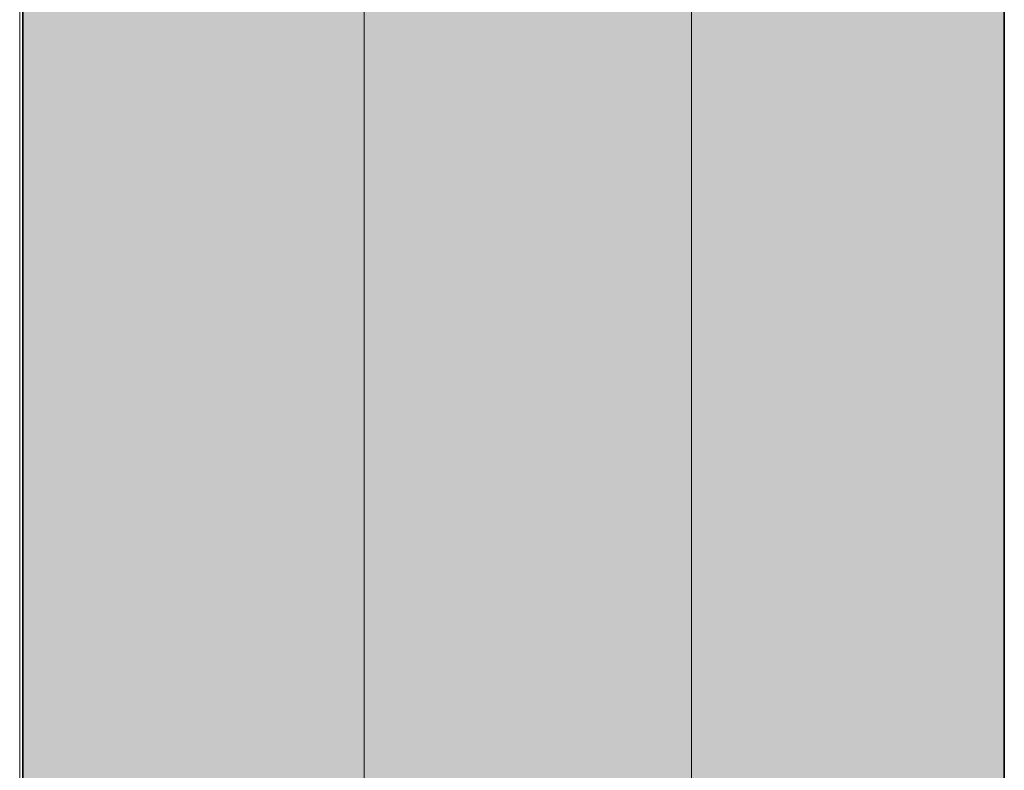
# Model space of a CAD drawing. Units: inches. Extents: x 2091 to 2899, y 967 to 2217.
# Tile 238 of 256: x 2203 to 2212, y 1159 to 1166. Entities that reach past the tile are written whole.
import ezdxf

# ---------------------------------------------------------------- set-up
doc = ezdxf.new("R2010")
doc.units = ezdxf.units.IN
for name, color, linetype, lineweight in [('A-GLAZ', 4, 'Continuous', 18), ('A-WALL', 7, 'Continuous', 35), ('C-PROP', 7, 'Continuous', 35)]:
    doc.layers.add(name, color=color, linetype=linetype, lineweight=lineweight)
doc.layers.add('A-WALL-PATT', color=141, linetype='Continuous', lineweight=13, true_color=0xadddf7)

# ---------------------------------------------------------------- blocks, each defined once
blk = doc.blocks.new('WIN-DOUBLE-LINE')
for p, q in [((0.0004, -0.0004), (0.0004, 80.8229)), ((3.1603, 80.8229), (3.1603, -0.0004)), ((6.1603, 80.8229), (6.1603, -0.0004))]:
    blk.add_line(p, q)

msp = doc.modelspace()

# ---------------------------------------------------------------- hatches: boundary and pattern name
at = {"layer": 'A-WALL-PATT'}
h = msp.add_hatch(color=256, dxfattribs=at)
h.dxf.hatch_style = 1
h.paths.add_polyline_path([(2803.1436, 2050.9191), (2203.1436, 2050.9191), (2203.1436, 1090.9191), (2803.1436, 1090.9191)])
h.paths.add_polyline_path([(2635.7989, 1147.5405), (2674.5241, 1147.5405, 0.376086), (2678.5297, 1152.8802), (2678.5297, 1159.5565, 0.333335), (2674.5243, 1163.5618), (2674.5243, 1163.5619), (2674.5243, 1192.9344), (2635.806, 1192.9344), (2597.0876, 1192.9344), (2597.0876, 1163.5618, 0.333335), (2593.0823, 1159.5565), (2593.0823, 1152.8802, 0.376086), (2597.0879, 1147.5405)], flags=0)
h.paths.add_polyline_path([(2436.0104, 1278.2408, 0.000483), (2435.9526, 1278.215, -0.001328), (2435.9356, 1278.1117, -0.001711), (2436.1164, 1278.0408, 0.002185)], flags=0)
h.paths.add_polyline_path([(2794.1436, 1143.4191), (2794.1436, 1347.4191), (2543.3702, 1347.4191), (2543.3702, 1351.9191), (2794.1436, 1351.9191), (2794.1436, 1392.7136), (2793.9474, 1392.7136), (2793.9474, 1473.5369), (2794.1436, 1473.5369), (2794.1436, 1531.9191), (2650.1436, 1531.9191), (2650.1436, 1536.4191), (2794.1436, 1536.4191), (2794.1436, 1692.4191), (2609.3756, 1692.4191), (2609.3756, 1644.4191), (2604.8756, 1644.4191), (2604.8756, 1744.9191), (2609.3756, 1744.9191), (2609.3756, 1696.9191), (2794.1436, 1696.9191), (2794.1436, 1780.9191), (2609.6436, 1780.9191), (2493.8756, 1780.9191), (2493.8756, 1785.4191), (2609.6436, 1785.4191), (2794.1436, 1785.4191), (2794.1436, 1847.9388), (2793.9512, 1847.9388), (2793.9512, 1928.7622), (2794.1436, 1928.7622), (2794.1436, 1941.4191), (2614.1436, 1941.4191), (2614.1436, 1821.4191), (2609.6436, 1821.4191), (2609.6436, 1941.4191), (2392.1436, 1941.4191), (2392.1436, 1819.9191), (2387.6436, 1819.9191), (2387.6436, 1941.4191), (2212.1436, 1941.4191), (2212.1436, 1783.9191), (2392.1436, 1783.9191), (2392.1436, 1780.9191), (2212.1436, 1780.9191), (2212.1436, 1629.4191), (2387.6436, 1629.4191), (2387.6436, 1744.9191), (2392.1436, 1744.9191), (2392.1436, 1627.9191), (2317.1436, 1627.9191), (2317.1436, 1551.4191), (2317.1436, 1536.4191), (2459.3836, 1536.4191), (2459.3836, 1602.3965), (2463.8836, 1602.3965), (2463.8836, 1531.9191), (2456.6436, 1531.9191), (2456.6436, 1529.9191), (2452.1436, 1529.9191), (2452.1436, 1531.9191), (2312.6436, 1531.9191), (2312.6436, 1551.4191), (2306.1436, 1551.4191), (2306.1436, 1555.9191), (2308.1436, 1555.9191), (2308.1436, 1551.4191), (2312.6436, 1551.4191), (2312.6436, 1627.9191), (2212.1436, 1627.9191), (2212.1436, 1555.9191), (2270.1436, 1555.9191), (2270.1436, 1551.4191), (2212.1436, 1551.4191), (2212.1436, 1351.9191), (2272.1436, 1351.9191), (2272.1436, 1347.4191), (2212.1436, 1347.4191), (2212.1436, 1275.4191), (2308.1436, 1275.4191), (2308.1436, 1351.9191), (2452.1436, 1351.9191), (2452.1436, 1493.9191), (2456.6436, 1493.9191), (2456.6436, 1347.4191), (2312.6436, 1347.4191), (2312.6436, 1270.9191), (2212.1436, 1270.9191), (2212.1436, 1099.9191), (2281.2375, 1099.9191), (2282.871, 1110.9138), (2282.0083, 1116.9966), (2278.5577, 1121.4204), (2268.2056, 1128.0562), (2272.0876, 1128.0562), (2273.8129, 1131.927), (2279.4203, 1134.6919), (2285.0278, 1135.2449), (2287.6158, 1137.4568), (2288.0471, 1138.0098), (2289.3411, 1140.7747), (2291.0665, 1139.6687), (2292.3605, 1135.2449), (2295.3798, 1136.9038), (2296.2425, 1135.7979), (2297.1052, 1133.033), (2300.1246, 1138.0098), (2303.1439, 1138.0098), (2304.4379, 1135.7979), (2303.1439, 1133.586), (2306.5946, 1134.6919), (2307.8887, 1133.033), (2310.908, 1135.2449), (2313.9274, 1134.1389), (2315.6269, 1132.4271), (2308.32, 1117.5496), (2290.2038, 1109.8079), (2288.9098, 1103.1721), (2289.2723, 1099.9191), (2434.9182, 1099.9191), (2431.5932, 1124.7881), (2429.9302, 1169.5531), (2430.9272, 1240.5197), (2435.6589, 1238.1861), (2437.1352, 1196.5541), (2438.7982, 1143.9731), (2442.6782, 1111.9981), (2446.5582, 1099.9191), (2794.1436, 1099.9191), (2794.1436, 1138.9191), (2548.0324, 1138.9191), (2548.0324, 1143.4191), (2548.0324, 1148.8191), (2546.6685, 1148.0316), (2528.6857, 1179.1786, 0.256256), (2512.0324, 1148.8191), (2512.0324, 1143.4191), (2512.0324, 1138.9191), (2507.5324, 1138.9191), (2507.5324, 1143.4191), (2507.5324, 1148.8191, 0.256256), (2490.8792, 1179.1786), (2472.8964, 1148.0316), (2471.5324, 1148.8191), (2471.5324, 1143.4191), (2467.0324, 1143.4191), (2467.0324, 1269.9458, 0.039061), (2460.91, 1273.5801), (2467.0324, 1273.5801), (2467.0324, 1286.3254, 0.014511), (2465.2162, 1286.7619), (2467.0324, 1287.0526), (2467.0324, 1323.4191), (2471.5324, 1323.4191), (2471.5324, 1148.8191), (2489.5324, 1179.996), (2490.8964, 1179.2085), (2490.8792, 1179.1786, -0.256256), (2507.5324, 1148.8191), (2507.5324, 1143.4191), (2512.0324, 1143.4191), (2512.0324, 1148.8191, -0.256256), (2528.6857, 1179.1786), (2528.6685, 1179.2085), (2530.0324, 1179.996), (2548.0324, 1148.8191), (2548.0324, 1143.4191)], flags=16)
h.paths.add_polyline_path([(2607.7685, 1200.9451), (2607.7685, 1265.0306), (2597.0876, 1281.052), (2619.7846, 1281.052), (2627.7953, 1337.1269), (2635.7989, 1337.1269), (2643.8167, 1337.1269), (2651.8274, 1281.052), (2674.5243, 1281.052), (2663.8434, 1265.0306), (2663.8434, 1200.9451), (2635.806, 1200.9451)], flags=0)
edge = h.paths.add_edge_path(flags=0)
edge.add_ellipse((13303.8962, 1272.9987), major_axis=(-10595.313, 0), ratio=0.8423038701, start_angle=0.62823722, end_angle=0.6465541, ccw=False)
edge.add_ellipse((2711.7004, 1156.8527), major_axis=(2.2198, 0), ratio=0.842304, start_angle=111.53524, end_angle=180.62824, ccw=False)
edge.add_ellipse((13303.1563, 1272.9987), major_axis=(-10593.0263, 0), ratio=0.8423038695, start_angle=0.52827147, end_angle=0.6465541, ccw=False)
edge.add_line((2710.7646, 1175.3333), (2710.13, 1175.3333))
edge.add_ellipse((2710.13, 1176.5798), major_axis=(1.4798, 0), ratio=0.842304, start_angle=180, end_angle=270, ccw=False)
edge.add_line((2708.6501, 1176.5798), (2708.6501, 1200.7829))
edge.add_ellipse((2710.13, 1200.7829), major_axis=(1.4798, 0), ratio=0.842304, start_angle=90, end_angle=180, ccw=False)
edge.add_line((2710.13, 1202.0294), (2710.4651, 1202.0294))
edge.add_ellipse((13303.1563, 1272.9987), major_axis=(-10593.0263, 0), ratio=0.8423038695, start_angle=-0.09022909, end_angle=0.38386678, ccw=False)
edge.add_ellipse((2710.13, 1290.927), major_axis=(-1.4798, 0), ratio=0.842304, start_angle=0, end_angle=90, ccw=False)
edge.add_line((2708.6501, 1290.927), (2708.6501, 1315.1302))
edge.add_ellipse((2710.13, 1315.1302), major_axis=(-1.4798, 0), ratio=0.842304, start_angle=-90, end_angle=0, ccw=False)
edge.add_line((2710.13, 1316.3767), (2710.7063, 1316.3767))
edge.add_ellipse((3238.4017, 1296.2896), major_axis=(528.234, 0), ratio=0.84230387, start_angle=176.349572, end_angle=177.82005, ccw=False)
edge.add_ellipse((2775.063, 1071.4507), major_axis=(313.3078, 0), ratio=0.84230387, start_angle=102.125966, end_angle=103.780529, ccw=False)
edge.add_ellipse((2775.063, 1078.3057), major_axis=(-305.3029, 0), ratio=0.84230387, start_angle=-79.790461, end_angle=-77.555373, ccw=False)
edge.add_ellipse((2695.1418, 1541.9754), major_axis=(-250.9602, 0), ratio=0.84230387, start_angle=99.256566, end_angle=102.554933)
edge.add_line((2741.4103, 1334.2143), (2747.1325, 1337.3785))
edge.add_ellipse((2747.5386, 1336.8575), major_axis=(-0.7399, 0), ratio=0.842304, start_angle=270, end_angle=307.93313, ccw=False)
edge.add_ellipse((2747.5386, 1336.8575), major_axis=(-0.7399, 0), ratio=0.842304, start_angle=232.06687, end_angle=270, ccw=False)
edge.add_line((2747.9447, 1337.3785), (2753.6669, 1334.2143))
edge.add_ellipse((2799.9355, 1541.9754), major_axis=(250.9602, 0), ratio=0.84230387, start_angle=257.445067, end_angle=260.743434)
edge.add_ellipse((2720.0142, 1078.3057), major_axis=(305.3029, 0), ratio=0.84230387, start_angle=77.555373, end_angle=79.790461, ccw=False)
edge.add_ellipse((2720.0142, 1071.4507), major_axis=(-313.3078, 0), ratio=0.84230387, start_angle=256.219471, end_angle=257.874034, ccw=False)
edge.add_ellipse((2256.6755, 1296.2896), major_axis=(-528.234, 0), ratio=0.84230387, start_angle=182.17995, end_angle=183.650428, ccw=False)
edge.add_line((2784.3709, 1316.3767), (2784.9472, 1316.3767))
edge.add_ellipse((2784.9472, 1315.1302), major_axis=(1.4798, 0), ratio=0.842304, start_angle=0, end_angle=90, ccw=False)
edge.add_line((2786.4271, 1315.1302), (2786.4271, 1290.927))
edge.add_ellipse((2784.9472, 1290.927), major_axis=(1.4798, 0), ratio=0.842304, start_angle=270, end_angle=360, ccw=False)
edge.add_ellipse((-7808.0791, 1272.9987), major_axis=(10593.0263, 0), ratio=0.8423038695, start_angle=-0.38386678, end_angle=0.09022909, ccw=False)
edge.add_line((2784.6122, 1202.0294), (2784.9472, 1202.0294))
edge.add_ellipse((2784.9472, 1200.7829), major_axis=(1.4798, 0), ratio=0.842304, start_angle=0, end_angle=90, ccw=False)
edge.add_line((2786.4271, 1200.7829), (2786.4271, 1176.5798))
edge.add_ellipse((2784.9472, 1176.5798), major_axis=(-1.4798, 0), ratio=0.842304, start_angle=90, end_angle=180, ccw=False)
edge.add_line((2784.9472, 1175.3333), (2784.3126, 1175.3333))
edge.add_ellipse((-7808.0791, 1272.9987), major_axis=(10593.0263, 0), ratio=0.8423038695, start_angle=-0.6186432, end_angle=-0.52827147, ccw=False)
edge.add_ellipse((2783.3768, 1156.8527), major_axis=(-2.2198, 0), ratio=0.842304, start_angle=179.37176, end_angle=248.46476, ccw=False)
edge.add_ellipse((-7808.819, 1272.9987), major_axis=(-10595.313, 0), ratio=0.8423038658, start_angle=179.35344592, end_angle=179.3717628, ccw=False)
edge.add_ellipse((2780.2973, 1153.5008), major_axis=(-5.2464, 0), ratio=0.842304, start_angle=90, end_angle=179.35345, ccw=False)
edge.add_line((2780.2973, 1149.0817), (2714.7799, 1149.0817))
edge.add_ellipse((2714.7799, 1153.5008), major_axis=(5.2464, 0), ratio=0.842304, start_angle=180.64655, end_angle=270, ccw=False)
edge = h.paths.add_edge_path(flags=0)
edge.add_line((2718.1874, 1151.0078), (2718.1874, 1170.4724))
edge.add_ellipse((2721.1471, 1170.4724), major_axis=(-2.9597, 0), ratio=0.842304, start_angle=-90, end_angle=0, ccw=False)
edge.add_line((2721.1471, 1172.9653), (2773.9302, 1172.9653))
edge.add_ellipse((2773.9302, 1170.4724), major_axis=(-2.9597, 0), ratio=0.842304, start_angle=180, end_angle=270, ccw=False)
edge.add_line((2776.8899, 1170.4724), (2776.8899, 1151.0078))
edge.add_line((2776.8899, 1151.0078), (2718.1874, 1151.0078))
edge = h.paths.add_edge_path(flags=0)
edge.add_line((2718.1874, 1180.2342), (2718.1874, 1199.0578))
edge.add_ellipse((2747.5386, 1320.3986), major_axis=(147.0179, 0), ratio=0.84230387, start_angle=256.401865, end_angle=283.598135)
edge.add_line((2776.8899, 1199.0578), (2776.8899, 1180.2342))
edge.add_ellipse((2747.5386, 1301.575), major_axis=(147.0179, 0), ratio=0.84230387, start_angle=256.401865, end_angle=283.598135, ccw=False)
edge = h.paths.add_edge_path(flags=0)
edge.add_ellipse((13303.1563, 1272.9987), major_axis=(-10591.5465, 0), ratio=0.8423038696, start_angle=0.05559431, end_angle=0.37776419, ccw=False)
edge.add_line((2711.6169, 1262.7217), (2715.6674, 1249.4954))
edge.add_ellipse((6413.892, 1241.6919), major_axis=(-3698.2362, 0), ratio=0.84230387, start_angle=-0.1208974, end_angle=0.3640763)
edge.add_line((2715.761, 1218.1925), (2711.9343, 1203.1674))
edge = h.paths.add_edge_path(flags=0)
edge.add_line((2718.1874, 1251.0746), (2716.0025, 1267.4504))
edge.add_ellipse((2742.1512, 1202.1895), major_axis=(81.7726, 0), ratio=0.8423039, start_angle=94.277421, end_angle=111.834954, ccw=False)
edge.add_line((2737.0097, 1270.9306), (2758.0675, 1270.9306))
edge.add_ellipse((2752.9261, 1202.1895), major_axis=(81.7726, 0), ratio=0.8423039, start_angle=68.165046, end_angle=85.722579, ccw=False)
edge.add_line((2779.0747, 1267.4504), (2776.8899, 1251.0746))
edge.add_ellipse((2750.3381, 1187.8854), major_axis=(79.5797, 0), ratio=0.8423039, start_angle=67.208085, end_angle=85.12993)
edge.add_line((2756.0347, 1254.7437), (2739.0426, 1254.7437))
edge.add_ellipse((2744.7392, 1187.8854), major_axis=(79.5797, 0), ratio=0.8423039, start_angle=94.87007, end_angle=112.791915)
edge = h.paths.add_edge_path(flags=0)
edge.add_line((2783.1429, 1203.1674), (2779.3162, 1218.1925))
edge.add_ellipse((-918.8147, 1241.6919), major_axis=(3698.2362, 0), ratio=0.84230387, start_angle=-0.3640763, end_angle=0.1208974)
edge.add_line((2779.4098, 1249.4954), (2783.4604, 1262.7217))
edge.add_ellipse((-7808.0791, 1272.9987), major_axis=(-10591.5465, 0), ratio=0.8423038695, start_angle=179.62223581, end_angle=179.94440569, ccw=False)
edge = h.paths.add_edge_path(flags=0)
edge.add_ellipse((2734.2009, 1286.6904), major_axis=(-0.3566, 6.3401), ratio=0.603834, start_angle=89.00201, end_angle=253.65741, ccw=False)
edge.add_line((2730.369, 1286.5418), (2730.369, 1301.352))
edge.add_line((2730.369, 1301.352), (2735.9133, 1305.2148))
edge.add_ellipse((2736.3849, 1304.7346), major_axis=(0.7399, 0), ratio=0.842304, start_angle=90, end_angle=134.48021, ccw=False)
edge.add_line((2736.3849, 1305.3578), (2738.0328, 1305.3578))
edge.add_line((2738.0328, 1305.3578), (2738.0328, 1307.7079))
edge.add_ellipse((2794.2016, 1307.7079), major_axis=(56.1689, 0), ratio=0.8423039, start_angle=150.56143, end_angle=180, ccw=False)
edge.add_ellipse((2700.8756, 1307.7079), major_axis=(-56.1689, 0), ratio=0.8423039, start_angle=180, end_angle=209.43857, ccw=False)
edge.add_line((2757.0444, 1307.7079), (2757.0444, 1305.3578))
edge.add_line((2757.0444, 1305.3578), (2758.6923, 1305.3578))
edge.add_ellipse((2758.6923, 1304.7346), major_axis=(-0.7399, 0), ratio=0.842304, start_angle=225.51979, end_angle=270, ccw=False)
edge.add_line((2759.1639, 1305.2148), (2764.7082, 1301.352))
edge.add_line((2764.7082, 1301.352), (2764.7082, 1286.5418))
edge.add_ellipse((2760.8763, 1286.6904), major_axis=(0.3566, 6.3401), ratio=0.603834, start_angle=106.34259, end_angle=270.99799, ccw=False)
edge.add_line((2757.0444, 1285.7971), (2757.0444, 1307.7079))
edge.add_ellipse((2700.8756, 1307.7079), major_axis=(-56.1689, 0), ratio=0.8423039, start_angle=180, end_angle=209.43857)
edge.add_ellipse((2794.2016, 1307.7079), major_axis=(56.1689, 0), ratio=0.8423039, start_angle=150.56143, end_angle=180)
edge.add_line((2738.0328, 1307.7079), (2738.0328, 1285.7971))
h.paths.add_polyline_path([(2417.8123, 1104.4497), (2413.4923, 1102.5297), (2410.6123, 1103.9697), (2409.1723, 1106.3697), (2407.2523, 1107.3297), (2406.2923, 1109.7297), (2405.3323, 1114.0497), (2405.3323, 1117.8897), (2406.2923, 1120.1297), (2407.2523, 1119.8097), (2408.8483, 1118.3277), (2410.1739, 1119.4242), (2410.2113, 1120.4057), (2411.0407, 1121.4191), (2410.6993, 1119.8587), (2410.1739, 1119.4242), (2410.0885, 1117.1761), (2411.1328, 1116.2063), (2413.9723, 1119.3297), (2416.8523, 1120.7697), (2416.8697, 1120.7988), (2417.0351, 1119.4051), (2417.8962, 1118.1434), (2418.2923, 1118.3697), (2419.5444, 1120.0393), (2419.3609, 1118.3875), (2419.0321, 1119.3562), (2418.3989, 1118.5119), (2419.2523, 1114.5297), (2418.7941, 1107.1988)], flags=0)
h.paths.add_polyline_path([(2508.8702, 1347.4191), (2508.3702, 1347.4191), (2508.3702, 1351.9191), (2508.8702, 1351.9191)], flags=0)
h.paths.add_polyline_path([(2473.3702, 1347.4191), (2472.3702, 1347.4191), (2467.8702, 1347.4191), (2467.8702, 1455.4191), (2472.3702, 1455.4191), (2472.3702, 1352.4191), (2473.3702, 1352.4191)], flags=0)
h.paths.add_polyline_path([(2352.1062, 1217.4462), (2349.2262, 1218.8862), (2347.7862, 1221.2862), (2345.8662, 1222.2462), (2344.9062, 1224.6462), (2343.9462, 1228.9662), (2343.9462, 1232.8062), (2344.9062, 1235.0462), (2345.8662, 1234.7262), (2347.4623, 1233.2442), (2348.7879, 1234.3407), (2348.8252, 1235.3222), (2349.6547, 1236.3355), (2349.3132, 1234.7752), (2348.7879, 1234.3407), (2348.7024, 1232.0926), (2349.7468, 1231.1228), (2352.5862, 1234.2462), (2355.4662, 1235.6862), (2355.4837, 1235.7153), (2355.649, 1234.3216), (2356.5102, 1233.0599), (2356.9062, 1233.2862), (2358.1584, 1234.9558), (2357.9749, 1233.304), (2357.6461, 1234.2726), (2357.0129, 1233.4284), (2357.8662, 1229.4462), (2357.4081, 1222.1153), (2356.4262, 1219.3662)], flags=0)
h.paths.add_polyline_path([(2348.2968, 1112.2244), (2347.0138, 1112.3104), (2345.5298, 1114.1274), (2345.7318, 1115.8584), (2346.8118, 1116.9824), (2346.8118, 1114.6464), (2345.8668, 1114.2144), (2346.8798, 1114.3004)], flags=0)
h.paths.add_polyline_path([(2347.0138, 1110.9264), (2346.2718, 1110.4934), (2346.6098, 1111.1864)], flags=0)
h.paths.add_polyline_path([(2345.8668, 1118.1944), (2345.5298, 1117.3294), (2343.7078, 1118.0214), (2344.3828, 1118.6264)], flags=0)
h.paths.add_polyline_path([(2346.6768, 1109.2824), (2346.0698, 1108.0714), (2345.8668, 1110.0614)], flags=0)
h.paths.add_polyline_path([(2345.0568, 1119.7514), (2343.6398, 1119.7514), (2343.9778, 1121.1354)], flags=0)
h.paths.add_polyline_path([(2345.2598, 1116.5504), (2345.1248, 1115.8584), (2344.9218, 1115.6854), (2344.7198, 1116.3774)], flags=0)
h.paths.add_polyline_path([(2345.6648, 1112.3104), (2345.4618, 1111.5324), (2344.0448, 1111.9644), (2344.6518, 1112.5704)], flags=0)
h.paths.add_polyline_path([(2345.1918, 1113.3494), (2344.4498, 1113.8684), (2344.7198, 1114.3874)], flags=0)
h.paths.add_polyline_path([(2344.6518, 1116.8094), (2344.1798, 1115.6854), (2344.6518, 1115.3394), (2343.9098, 1114.9064), (2343.0328, 1115.9444), (2343.6398, 1116.4634)], flags=0)
h.paths.add_polyline_path([(2345.8668, 1106.6864), (2344.9898, 1105.5624), (2344.5168, 1106.6004)], flags=0)
h.paths.add_polyline_path([(2344.8548, 1110.0614), (2344.5168, 1109.2824), (2344.1128, 1109.7154)], flags=0)
h.paths.add_polyline_path([(2344.0448, 1113.5224), (2343.4378, 1113.0894), (2342.7628, 1113.9544)], flags=0)
h.paths.add_polyline_path([(2344.3148, 1111.0124), (2342.9648, 1110.3204), (2342.9648, 1111.0994)], flags=0)
h.paths.add_polyline_path([(2345.1248, 1104.6974), (2344.5848, 1103.7454), (2344.4498, 1104.2644)], flags=0)
h.paths.add_polyline_path([(2342.8298, 1121.2224), (2341.7498, 1120.5304), (2340.5358, 1121.0494), (2340.1308, 1121.8284), (2340.6708, 1122.9524), (2341.1428, 1121.8284), (2341.6148, 1122.0014)], flags=0)
h.paths.add_polyline_path([(2342.9648, 1119.7514), (2343.0328, 1118.4534), (2342.0878, 1118.0214), (2342.0198, 1119.4914)], flags=0)
h.paths.add_polyline_path([(2342.6948, 1116.8964), (2341.9528, 1116.6364), (2342.0198, 1117.3294)], flags=0)
h.paths.add_polyline_path([(2343.0328, 1112.2244), (2342.0198, 1111.7914), (2341.5478, 1112.2244), (2342.3578, 1113.3494)], flags=0)
h.paths.add_polyline_path([(2343.7748, 1104.4374), (2342.6278, 1102.8804), (2342.6948, 1104.6104), (2343.4378, 1105.1294)], flags=0)
h.paths.add_polyline_path([(2342.0198, 1115.0794), (2340.8058, 1115.5124), (2340.9408, 1116.3774)], flags=0)
h.paths.add_polyline_path([(2341.4808, 1120.0974), (2341.4808, 1119.4054), (2341.0758, 1119.5784), (2341.1428, 1120.0974)], flags=0)
h.paths.add_polyline_path([(2341.8178, 1114.4734), (2340.9408, 1113.0894), (2340.8058, 1114.5604)], flags=0)
h.paths.add_polyline_path([(2341.1428, 1118.5404), (2340.9408, 1116.9824), (2339.0508, 1117.6754), (2339.0508, 1118.6264)], flags=0)
h.paths.add_polyline_path([(2342.6948, 1101.6684), (2341.9528, 1101.8414), (2342.5598, 1102.3614)], flags=0)
h.paths.add_polyline_path([(2340.3328, 1119.6654), (2338.4438, 1119.5784), (2337.9038, 1120.3574), (2339.6578, 1120.6164)], flags=0)
h.paths.add_polyline_path([(2340.3328, 1115.3394), (2340.0628, 1113.6954), (2339.3878, 1115.3394)], flags=0)
h.paths.add_polyline_path([(2341.8178, 1103.8314), (2341.5478, 1102.8804), (2341.1428, 1103.6584)], flags=0)
h.paths.add_polyline_path([(2339.0508, 1122.8664), (2337.2958, 1121.8284), (2337.0938, 1123.1254), (2337.7688, 1123.8184)], flags=0)
h.paths.add_polyline_path([(2339.1178, 1121.7414), (2338.8478, 1121.2224), (2338.1738, 1121.0494), (2338.3758, 1121.5684)], flags=0)
h.paths.add_polyline_path([(2339.1858, 1119.3194), (2338.6458, 1118.7134), (2338.2408, 1118.1074), (2338.2408, 1118.8864)], flags=0)
h.paths.add_polyline_path([(2341.1428, 1101.9284), (2340.6028, 1101.2364), (2340.0628, 1101.8414), (2340.6028, 1102.3614)], flags=0)
h.paths.add_polyline_path([(2337.6338, 1117.7614), (2336.6208, 1118.2804), (2337.2958, 1118.9724)], flags=0)
h.paths.add_polyline_path([(2336.8238, 1119.5784), (2334.7988, 1118.9724), (2335.2038, 1120.3574), (2336.5538, 1120.8764)], flags=0)
h.paths.add_polyline_path([(2339.1178, 1100.4574), (2337.3638, 1100.5434), (2336.7558, 1101.2364)], flags=0)
h.paths.add_polyline_path([(2336.3508, 1122.4334), (2336.0138, 1121.9144), (2334.9338, 1122.4334), (2334.5288, 1123.4714), (2335.7438, 1122.7794)], flags=0)
h.paths.add_polyline_path([(2334.7318, 1120.8764), (2334.2588, 1120.3574), (2334.0568, 1120.7894), (2334.5968, 1121.3084)], flags=0)
h.paths.add_polyline_path([(2334.4618, 1122.1744), (2332.5718, 1121.3084), (2331.3568, 1122.1744), (2332.0998, 1122.8664)], flags=0)
h.paths.add_polyline_path([(2334.2588, 1118.5404), (2333.3818, 1118.4534), (2333.6518, 1119.3194)], flags=0)
h.paths.add_polyline_path([(2335.5418, 1102.2744), (2334.1918, 1102.6204), (2335.2718, 1103.3124)], flags=0)
h.paths.add_polyline_path([(2332.7068, 1119.6654), (2331.6948, 1120.4434), (2332.5048, 1120.7894)], flags=0)
h.paths.add_polyline_path([(2334.7318, 1101.1494), (2333.5168, 1101.5824), (2333.9888, 1101.7554)], flags=0)
h.paths.add_polyline_path([(2332.6398, 1116.6364), (2331.0868, 1116.2904), (2331.9648, 1118.1944)], flags=0)
h.paths.add_polyline_path([(2330.7498, 1121.5684), (2330.2768, 1120.2704), (2328.5228, 1119.3194), (2328.9948, 1121.0494)], flags=0)
h.paths.add_polyline_path([(2330.7498, 1118.6264), (2330.0078, 1117.5024), (2329.8728, 1118.0214)], flags=0)
h.paths.add_polyline_path([(2332.0998, 1102.3614), (2330.5468, 1102.0144), (2331.6948, 1102.9664)], flags=0)
h.paths.add_polyline_path([(2329.5348, 1113.6084), (2329.0628, 1112.3104), (2328.5898, 1113.3494)], flags=0)
h.paths.add_polyline_path([(2328.3878, 1117.8484), (2327.5098, 1116.5504), (2327.1728, 1117.7614)], flags=0)
h.paths.add_polyline_path([(2329.7378, 1106.5134), (2329.5348, 1105.3024), (2328.2528, 1106.0814)], flags=0)
h.paths.add_polyline_path([(2328.6578, 1114.3874), (2328.0498, 1114.1274), (2328.3198, 1114.9064)], flags=0)
h.paths.add_polyline_path([(2328.3198, 1112.2244), (2327.1058, 1112.1374), (2326.7008, 1112.6564)], flags=0)
h.paths.add_polyline_path([(2326.9028, 1115.2524), (2326.7008, 1114.1274), (2325.2158, 1113.6084), (2326.0928, 1115.3394)], flags=0)
h.paths.add_polyline_path([(2326.6328, 1108.3304), (2326.0928, 1107.3794), (2325.8908, 1108.5034), (2326.4978, 1109.1094)], flags=0)
h.paths.add_polyline_path([(2615.1436, 1531.9191), (2609.6436, 1531.9191), (2609.6436, 1620.4191), (2614.1436, 1620.4191), (2614.1436, 1536.4191), (2615.1436, 1536.4191)], flags=0)
h.paths.add_polyline_path([(2545.1436, 1563.4191), (2464.1436, 1563.4191), (2464.1436, 1632.4191), (2509.1436, 1632.4191), (2509.1436, 1627.9191), (2509.1436, 1603.9191), (2468.6436, 1603.9191), (2468.6436, 1567.9191), (2540.6436, 1567.9191), (2540.6436, 1591.9191), (2545.1436, 1591.9191)], flags=0)
h.paths.add_polyline_path([(2388.969, 1549.9857), (2357.4342, 1549.9857), (2357.4342, 1623.3608), (2399.3628, 1623.3608), (2435.6895, 1623.3608), (2435.5925, 1602.5593), (2435.5925, 1602.3965), (2388.969, 1602.3965)], flags=0)
h.paths.add_polyline_path([(2388.8806, 1555.8092), (2374.9044, 1555.8092), (2374.9044, 1600.5716), (2374.9044, 1615.4576), (2406.3509, 1615.4576), (2406.3509, 1618.9394), (2412.1743, 1615.4576), (2406.3509, 1611.9759), (2406.3509, 1615.4576), (2388.8806, 1615.4576)], flags=0)
h.paths.add_polyline_path([(2568.8756, 1644.4191), (2453.3756, 1644.4191), (2453.3756, 1785.4191), (2457.8756, 1785.4191), (2457.8756, 1648.9191), (2568.8756, 1648.9191)], flags=0)
h.paths.add_polyline_path([(2212.1436, 1945.9191), (2212.1436, 2041.9191), (2794.1436, 2041.9191), (2794.1436, 1945.9191)], flags=16)
h.paths.add_polyline_path([(2271.0827, 1964.3172), (2776.853, 1964.3172), (2776.853, 2037.1696), (2271.0827, 2037.1696)], flags=8)
h.paths.add_polyline_path([(2380.6493, 1536.8241), (2461.0408, 1536.8241), (2461.0408, 1554.6526), (2380.6493, 1554.6526)], flags=8)
h.paths.add_polyline_path([(2240.7557, 1609.7255), (2309.1858, 1609.7255), (2309.1858, 1617.6982), (2240.7557, 1617.6982)], flags=8)
h.paths.add_polyline_path([(2212.6773, 1313.5041), (2282.5915, 1313.5041), (2282.5915, 1322.7452), (2212.6773, 1322.7452)], flags=8)
h.paths.add_polyline_path([(2457.112, 1114.7786), (2558.4816, 1114.7786), (2558.4816, 1142.2197), (2457.112, 1142.2197)], flags=8)
h.paths.add_polyline_path([(2473.4423, 1273.0101), (2604.6412, 1273.0101), (2604.6412, 1318.3469), (2473.4423, 1318.3469)], flags=8)
h.paths.add_polyline_path([(2638.8763, 1626.9774), (2684.2504, 1627.9767), (2684.0385, 1637.5975), (2638.6644, 1636.5982)], flags=8)
h.paths.add_polyline_path([(2537.5906, 1453.7934), (2628.3895, 1453.7934), (2628.3895, 1475.3448), (2537.5906, 1475.3448)], flags=8)
h.paths.add_polyline_path([(2504.1376, 1714.6324), (2554.6472, 1714.6324), (2554.6472, 1730.2377), (2504.1376, 1730.2377)], flags=8)
h.paths.add_polyline_path([(2487.5012, 1575.6519), (2535.0971, 1575.6519), (2535.0971, 1598.3776), (2487.5012, 1598.3776)], flags=8)
h.paths.add_polyline_path([(2709.0994, 1735.7103), (2740.0166, 1735.7103), (2740.0166, 1749.9376), (2709.0994, 1749.9376)], flags=8)
h.paths.add_polyline_path([(2442.4384, 1792.1717), (2564.7288, 1792.1717), (2564.7288, 1842.0002), (2442.4384, 1842.0002)], flags=8)
h.paths.add_polyline_path([(2655.8158, 1809.6441), (2789.5201, 1806.6938), (2790.085, 1832.2916), (2656.3806, 1835.2419)], flags=8)
h.paths.add_polyline_path([(2234.8427, 1797.7201), (2368.5929, 1794.7689), (2369.1607, 1820.5041), (2235.4106, 1823.4554)], flags=8)
h.paths.add_polyline_path([(2245.1385, 1644.0063), (2398.4277, 1640.6239), (2398.9948, 1666.3248), (2245.7056, 1669.7073)], flags=8)
h.paths.add_polyline_path([(2306.1428, 1431.1685), (2413.7683, 1428.7937), (2414.3331, 1454.3915), (2306.7077, 1456.7664)], flags=8)
h.paths.add_polyline_path([(2306.8346, 1458.2331), (2393.3805, 1456.3234), (2393.9328, 1481.3544), (2307.3869, 1483.2641)], flags=8)

# ---------------------------------------------------------------- linework, layer by layer
at = {"layer": 'A-WALL'}
msp.add_line((2212.1436, 1099.9191), (2212.1436, 1627.9191), dxfattribs=at)
at = {"layer": 'C-PROP'}
msp.add_lwpolyline([(2203.1436, 2050.9191), (2803.1436, 2050.9191), (2803.1436, 1090.9191), (2203.1436, 1090.9191)], close=True, dxfattribs=at)

# ---------------------------------------------------------------- block references
at = {"layer": 'A-GLAZ'}
msp.add_blockref('WIN-DOUBLE-LINE', (2203.1153, 1152.2475), dxfattribs=at)

doc.saveas('drawing.dxf')
